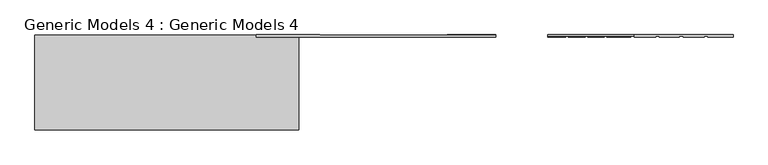
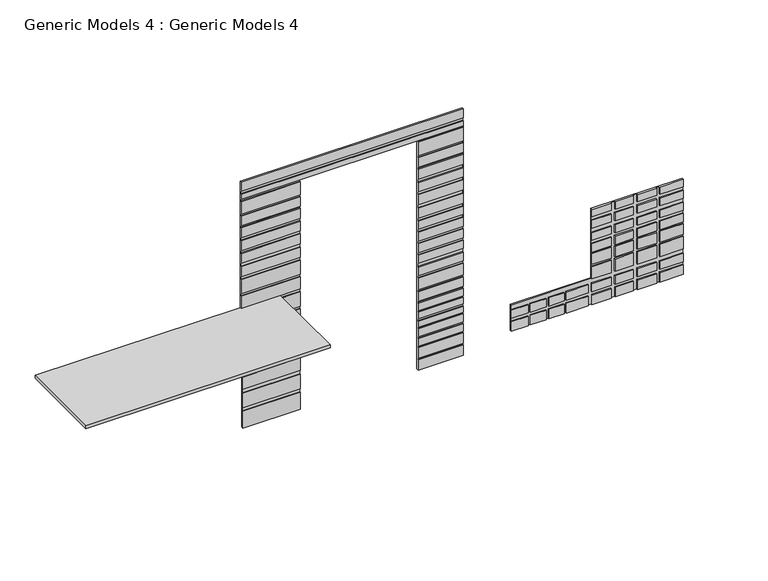
"""IFC4 building model written with IfcOpenShell, lengths in millimetres: proxy geometry, Generic Models 4 : Generic Models 4."""

from ifc_helpers import new_model, si_unit, origin, place, context, project, spatial, faceted_brep, source, transform, mapped, element, save


def generic_models_4_generic_models_4_6a6385c3(model_context):
    return source(origin(), model_context, "Body", "Brep", [
        faceted_brep([(-5873.014323, -13904.9538163, 2677.4848502), (-5873.014323, -13904.9538163, 2489.9387653), (-5393.446906, -13904.9538163, 2489.9387653), (-5393.446906, -13904.9538163, 2677.4848502), (-5873.014323, -13904.9538163, 2393.7857703), (-5873.014323, -13904.9538163, 2187.7436382), (-5393.446906, -13904.9538163, 2187.7436382), (-5393.446906, -13904.9538163, 2393.7857703), (-5873.014323, -13904.9538163, 2077.854501), (-5873.014323, -13904.9538163, 1876.5546729), (-5393.446906, -13904.9538163, 1876.5546729), (-5393.446906, -13904.9538163, 2077.854501), (-5873.014323, -13904.9538163, 1789.395516), (-5873.014323, -13904.9538163, 1569.6172418), (-5393.446906, -13904.9538163, 1569.6172418), (-5393.446906, -13904.9538163, 1789.395516), (-5873.014323, -13904.9538163, 1193.0039496), (-5873.014323, -13904.9538163, 872.4244956), (-5393.446906, -13904.9538163, 872.4244956), (-5393.446906, -13904.9538163, 1193.0039496), (-5873.014323, -13904.9538163, 1524.0), (-5873.014323, -13904.9538163, 1250.1296825), (-5393.446906, -13904.9538163, 1250.1296825), (-5393.446906, -13904.9538163, 1524.0), (-7854.214323, -13904.9538163, 455.5626701), (-7854.214323, -13904.9538163, 207.9039867), (-7441.5943921, -13904.9538163, 207.9039867), (-7441.5943921, -13904.9538163, 455.5626701), (-7854.214323, -13904.9538163, 753.9093053), (-7854.214323, -13904.9538163, 540.1642411), (-7441.5943921, -13904.9538163, 540.1642411), (-7441.5943921, -13904.9538163, 753.9093053), (-3625.114323, -13904.9538163, 2489.9387653), (-3625.114323, -13904.9538163, 2677.4848502), (-4204.9719989, -13904.9538163, 2677.4848502), (-4204.9719989, -13904.9538163, 2489.9387653), (-3625.114323, -13904.9538163, 2187.7436382), (-3625.114323, -13904.9538163, 2393.7857703), (-4204.9719989, -13904.9538163, 2393.7857703), (-4204.9719989, -13904.9538163, 2187.7436382), (-3625.114323, -13904.9538163, 1876.5546729), (-3625.114323, -13904.9538163, 2077.854501), (-4204.9719989, -13904.9538163, 2077.854501), (-4204.9719989, -13904.9538163, 1876.5546729), (-3625.114323, -13904.9538163, 1569.6172418), (-3625.114323, -13904.9538163, 1789.395516), (-4204.9719989, -13904.9538163, 1789.395516), (-4204.9719989, -13904.9538163, 1569.6172418), (-3625.114323, -13904.9538163, 872.4244956), (-3625.114323, -13904.9538163, 1193.0039496), (-4204.9719989, -13904.9538163, 1193.0039496), (-4204.9719989, -13904.9538163, 872.4244956), (-3625.114323, -13904.9538163, 1250.1296825), (-3625.114323, -13904.9538163, 1524.0), (-4204.9719989, -13904.9538163, 1524.0), (-4204.9719989, -13904.9538163, 1250.1296825), (-3625.114323, -13904.9538163, 207.9039867), (-3625.114323, -13904.9538163, 455.5626701), (-4204.9719989, -13904.9538163, 455.5626701), (-4204.9719989, -13904.9538163, 207.9039867), (-3625.114323, -13904.9538163, 540.1642411), (-3625.114323, -13904.9538163, 753.9093053), (-4204.9719989, -13904.9538163, 753.9093053), (-4204.9719989, -13904.9538163, 540.1642411), (-4855.9456918, -13904.9538163, 2677.4848502), (-5303.8633703, -13904.9538163, 2677.4848502), (-5303.8633703, -13904.9538163, 2489.9387653), (-4855.9456918, -13904.9538163, 2489.9387653), (-4282.6110632, -13904.9538163, 2677.4848502), (-4760.3899203, -13904.9538163, 2677.4848502), (-4760.3899203, -13904.9538163, 2489.9387653), (-4282.6110632, -13904.9538163, 2489.9387653), (-5303.8633703, -13904.9538163, 207.9039867), (-4855.9456918, -13904.9538163, 207.9039867), (-4855.9456918, -13904.9538163, 455.5626701), (-5303.8633703, -13904.9538163, 455.5626701), (-4760.3899203, -13904.9538163, 207.9039867), (-4282.6110632, -13904.9538163, 207.9039867), (-4282.6110632, -13904.9538163, 455.5626701), (-4760.3899203, -13904.9538163, 455.5626701), (-5873.014323, -13904.9538163, 207.9039867), (-5393.446906, -13904.9538163, 207.9039867), (-5393.446906, -13904.9538163, 455.5626701), (-5873.014323, -13904.9538163, 455.5626701), (-6501.664323, -13904.9538163, 207.9039867), (-5956.9143625, -13904.9538163, 207.9039867), (-5956.9143625, -13904.9538163, 455.5626701), (-6501.664323, -13904.9538163, 455.5626701), (-6935.8171521, -13904.9538163, 207.9039867), (-6556.6805641, -13904.9538163, 207.9039867), (-6556.6805641, -13904.9538163, 455.5626701), (-6935.8171521, -13904.9538163, 455.5626701), (-7382.8881053, -13904.9538163, 207.9039867), (-6999.0393071, -13904.9538163, 207.9039867), (-6999.0393071, -13904.9538163, 455.5626701), (-7382.8881053, -13904.9538163, 455.5626701), (-5303.8633703, -13904.9538163, 2187.7436382), (-4855.9456918, -13904.9538163, 2187.7436382), (-4855.9456918, -13904.9538163, 2393.7857703), (-5303.8633703, -13904.9538163, 2393.7857703), (-4760.3899203, -13904.9538163, 2187.7436382), (-4282.6110632, -13904.9538163, 2187.7436382), (-4282.6110632, -13904.9538163, 2393.7857703), (-4760.3899203, -13904.9538163, 2393.7857703), (-5303.8633703, -13904.9538163, 1876.5546729), (-4855.9456918, -13904.9538163, 1876.5546729), (-4855.9456918, -13904.9538163, 2077.854501), (-5303.8633703, -13904.9538163, 2077.854501), (-4760.3899203, -13904.9538163, 1876.5546729), (-4282.6110632, -13904.9538163, 1876.5546729), (-4282.6110632, -13904.9538163, 2077.854501), (-4760.3899203, -13904.9538163, 2077.854501), (-5303.8633703, -13904.9538163, 1569.6172418), (-4855.9456918, -13904.9538163, 1569.6172418), (-4855.9456918, -13904.9538163, 1789.395516), (-5303.8633703, -13904.9538163, 1789.395516), (-4760.3899203, -13904.9538163, 1569.6172418), (-4282.6110632, -13904.9538163, 1569.6172418), (-4282.6110632, -13904.9538163, 1789.395516), (-4760.3899203, -13904.9538163, 1789.395516), (-5303.8633703, -13904.9538163, 872.4244956), (-4855.9456918, -13904.9538163, 872.4244956), (-4855.9456918, -13904.9538163, 1193.0039496), (-5303.8633703, -13904.9538163, 1193.0039496), (-4760.3899203, -13904.9538163, 872.4244956), (-4282.6110632, -13904.9538163, 872.4244956), (-4282.6110632, -13904.9538163, 1193.0039496), (-4760.3899203, -13904.9538163, 1193.0039496), (-5303.8633703, -13904.9538163, 1250.1296825), (-4855.9456918, -13904.9538163, 1250.1296825), (-4855.9456918, -13904.9538163, 1524.0), (-5303.8633703, -13904.9538163, 1524.0), (-4760.3899203, -13904.9538163, 1250.1296825), (-4282.6110632, -13904.9538163, 1250.1296825), (-4282.6110632, -13904.9538163, 1524.0), (-4760.3899203, -13904.9538163, 1524.0), (-5303.8633703, -13904.9538163, 540.1642411), (-4855.9456918, -13904.9538163, 540.1642411), (-4855.9456918, -13904.9538163, 753.9093053), (-5303.8633703, -13904.9538163, 753.9093053), (-4760.3899203, -13904.9538163, 540.1642411), (-4282.6110632, -13904.9538163, 540.1642411), (-4282.6110632, -13904.9538163, 753.9093053), (-4760.3899203, -13904.9538163, 753.9093053), (-5873.014323, -13904.9538163, 540.1642411), (-5393.446906, -13904.9538163, 540.1642411), (-5393.446906, -13904.9538163, 753.9093053), (-5873.014323, -13904.9538163, 753.9093053), (-6501.664323, -13904.9538163, 540.1642411), (-5956.9143625, -13904.9538163, 540.1642411), (-5956.9143625, -13904.9538163, 753.9093053), (-6501.664323, -13904.9538163, 753.9093053), (-6935.8171521, -13904.9538163, 540.1642411), (-6556.6805641, -13904.9538163, 540.1642411), (-6556.6805641, -13904.9538163, 753.9093053), (-6935.8171521, -13904.9538163, 753.9093053), (-7382.8881053, -13904.9538163, 540.1642411), (-6999.0393071, -13904.9538163, 540.1642411), (-6999.0393071, -13904.9538163, 753.9093053), (-7382.8881053, -13904.9538163, 753.9093053), (-3625.114323, -13854.1538163, 2677.4848502), (-3625.114323, -13854.1538163, 207.9039867), (-7854.214323, -13854.1538163, 207.9039867), (-7854.214323, -13854.1538163, 872.4244956), (-5873.014323, -13854.1538163, 872.4244956), (-5873.014323, -13854.1538163, 2677.4848502), (-5393.446906, -13879.5538163, 2677.4848502), (-5303.8633703, -13879.5538163, 2677.4848502), (-4855.9456918, -13879.5538163, 2677.4848502), (-4760.3899203, -13879.5538163, 2677.4848502), (-4282.6110632, -13879.5538163, 2677.4848502), (-4204.9719989, -13879.5538163, 2677.4848502), (-5873.014323, -13879.5538163, 872.4244956), (-5873.014323, -13879.5538163, 1193.0039496), (-5873.014323, -13879.5538163, 1250.1296825), (-5873.014323, -13879.5538163, 1524.0), (-5873.014323, -13879.5538163, 1569.6172418), (-5873.014323, -13879.5538163, 1789.395516), (-5873.014323, -13879.5538163, 1876.5546729), (-5873.014323, -13879.5538163, 2077.854501), (-5873.014323, -13879.5538163, 2187.7436382), (-5873.014323, -13879.5538163, 2393.7857703), (-5873.014323, -13879.5538163, 2489.9387653), (-4204.9719989, -13879.5538163, 207.9039867), (-4282.6110632, -13879.5538163, 207.9039867), (-4760.3899203, -13879.5538163, 207.9039867), (-4855.9456918, -13879.5538163, 207.9039867), (-5303.8633703, -13879.5538163, 207.9039867), (-5393.446906, -13879.5538163, 207.9039867), (-5873.014323, -13879.5538163, 207.9039867), (-5956.9143625, -13879.5538163, 207.9039867), (-6501.664323, -13879.5538163, 207.9039867), (-6556.6805641, -13879.5538163, 207.9039867), (-6935.8171521, -13879.5538163, 207.9039867), (-6999.0393071, -13879.5538163, 207.9039867), (-7382.8881053, -13879.5538163, 207.9039867), (-7441.5943921, -13879.5538163, 207.9039867), (-3625.114323, -13879.5538163, 2489.9387653), (-3625.114323, -13879.5538163, 2393.7857703), (-3625.114323, -13879.5538163, 2187.7436382), (-3625.114323, -13879.5538163, 2077.854501), (-3625.114323, -13879.5538163, 1876.5546729), (-3625.114323, -13879.5538163, 1789.395516), (-3625.114323, -13879.5538163, 1569.6172418), (-3625.114323, -13879.5538163, 1524.0), (-3625.114323, -13879.5538163, 1250.1296825), (-3625.114323, -13879.5538163, 1193.0039496), (-3625.114323, -13879.5538163, 872.4244956), (-3625.114323, -13879.5538163, 753.9093053), (-3625.114323, -13879.5538163, 540.1642411), (-3625.114323, -13879.5538163, 455.5626701), (-7854.214323, -13879.5538163, 455.5626701), (-7854.214323, -13879.5538163, 540.1642411), (-7854.214323, -13879.5538163, 753.9093053), (-7854.214323, -13879.5538163, 872.4244956), (-5393.446906, -13879.5538163, 2393.7857703), (-5393.446906, -13879.5538163, 2187.7436382), (-5393.446906, -13879.5538163, 2077.854501), (-5393.446906, -13879.5538163, 1876.5546729), (-5393.446906, -13879.5538163, 1789.395516), (-5393.446906, -13879.5538163, 1569.6172418), (-5393.446906, -13879.5538163, 1524.0), (-5393.446906, -13879.5538163, 1250.1296825), (-5393.446906, -13879.5538163, 1193.0039496), (-5393.446906, -13879.5538163, 872.4244956), (-7441.5943921, -13879.5538163, 753.9093053), (-7441.5943921, -13879.5538163, 540.1642411), (-7441.5943921, -13879.5538163, 455.5626701), (-7382.8881053, -13879.5538163, 455.5626701), (-6999.0393071, -13879.5538163, 455.5626701), (-6935.8171521, -13879.5538163, 455.5626701), (-6556.6805641, -13879.5538163, 455.5626701), (-6501.664323, -13879.5538163, 455.5626701), (-5956.9143625, -13879.5538163, 455.5626701), (-5873.014323, -13879.5538163, 455.5626701), (-5393.446906, -13879.5538163, 455.5626701), (-5303.8633703, -13879.5538163, 455.5626701), (-4855.9456918, -13879.5538163, 455.5626701), (-4760.3899203, -13879.5538163, 455.5626701), (-4282.6110632, -13879.5538163, 455.5626701), (-4204.9719989, -13879.5538163, 455.5626701), (-4204.9719989, -13879.5538163, 540.1642411), (-4204.9719989, -13879.5538163, 753.9093053), (-4204.9719989, -13879.5538163, 872.4244956), (-4204.9719989, -13879.5538163, 1193.0039496), (-4204.9719989, -13879.5538163, 1250.1296825), (-4204.9719989, -13879.5538163, 1524.0), (-4204.9719989, -13879.5538163, 1569.6172418), (-4204.9719989, -13879.5538163, 1789.395516), (-4204.9719989, -13879.5538163, 1876.5546729), (-4204.9719989, -13879.5538163, 2077.854501), (-4204.9719989, -13879.5538163, 2187.7436382), (-4204.9719989, -13879.5538163, 2393.7857703), (-4204.9719989, -13879.5538163, 2489.9387653), (-4282.6110632, -13879.5538163, 2489.9387653), (-4760.3899203, -13879.5538163, 2489.9387653), (-4855.9456918, -13879.5538163, 2489.9387653), (-5303.8633703, -13879.5538163, 2489.9387653), (-5393.446906, -13879.5538163, 2489.9387653), (-5303.8633703, -13879.5538163, 2393.7857703), (-4855.9456918, -13879.5538163, 2393.7857703), (-4855.9456918, -13879.5538163, 2187.7436382), (-5303.8633703, -13879.5538163, 2187.7436382), (-4760.3899203, -13879.5538163, 2393.7857703), (-4282.6110632, -13879.5538163, 2393.7857703), (-4282.6110632, -13879.5538163, 2187.7436382), (-4760.3899203, -13879.5538163, 2187.7436382), (-5303.8633703, -13879.5538163, 2077.854501), (-4855.9456918, -13879.5538163, 2077.854501), (-4855.9456918, -13879.5538163, 1876.5546729), (-5303.8633703, -13879.5538163, 1876.5546729), (-4760.3899203, -13879.5538163, 2077.854501), (-4282.6110632, -13879.5538163, 2077.854501), (-4282.6110632, -13879.5538163, 1876.5546729), (-4760.3899203, -13879.5538163, 1876.5546729), (-5303.8633703, -13879.5538163, 1789.395516), (-4855.9456918, -13879.5538163, 1789.395516), (-4855.9456918, -13879.5538163, 1569.6172418), (-5303.8633703, -13879.5538163, 1569.6172418), (-4760.3899203, -13879.5538163, 1789.395516), (-4282.6110632, -13879.5538163, 1789.395516), (-4282.6110632, -13879.5538163, 1569.6172418), (-4760.3899203, -13879.5538163, 1569.6172418), (-5303.8633703, -13879.5538163, 1524.0), (-4855.9456918, -13879.5538163, 1524.0), (-4855.9456918, -13879.5538163, 1250.1296825), (-5303.8633703, -13879.5538163, 1250.1296825), (-4760.3899203, -13879.5538163, 1524.0), (-4282.6110632, -13879.5538163, 1524.0), (-4282.6110632, -13879.5538163, 1250.1296825), (-4760.3899203, -13879.5538163, 1250.1296825), (-5303.8633703, -13879.5538163, 753.9093053), (-4855.9456918, -13879.5538163, 753.9093053), (-4855.9456918, -13879.5538163, 540.1642411), (-5303.8633703, -13879.5538163, 540.1642411), (-4760.3899203, -13879.5538163, 753.9093053), (-4282.6110632, -13879.5538163, 753.9093053), (-4282.6110632, -13879.5538163, 540.1642411), (-4760.3899203, -13879.5538163, 540.1642411), (-5873.014323, -13879.5538163, 753.9093053), (-5393.446906, -13879.5538163, 753.9093053), (-5393.446906, -13879.5538163, 540.1642411), (-5873.014323, -13879.5538163, 540.1642411), (-6501.664323, -13879.5538163, 753.9093053), (-5956.9143625, -13879.5538163, 753.9093053), (-5956.9143625, -13879.5538163, 540.1642411), (-6501.664323, -13879.5538163, 540.1642411), (-6935.8171521, -13879.5538163, 753.9093053), (-6556.6805641, -13879.5538163, 753.9093053), (-6556.6805641, -13879.5538163, 540.1642411), (-6935.8171521, -13879.5538163, 540.1642411), (-7382.8881053, -13879.5538163, 753.9093053), (-6999.0393071, -13879.5538163, 753.9093053), (-6999.0393071, -13879.5538163, 540.1642411), (-7382.8881053, -13879.5538163, 540.1642411), (-5303.8633703, -13879.5538163, 1193.0039496), (-4855.9456918, -13879.5538163, 1193.0039496), (-4855.9456918, -13879.5538163, 872.4244956), (-5303.8633703, -13879.5538163, 872.4244956), (-4760.3899203, -13879.5538163, 1193.0039496), (-4282.6110632, -13879.5538163, 1193.0039496), (-4282.6110632, -13879.5538163, 872.4244956), (-4760.3899203, -13879.5538163, 872.4244956)], [[[0, 1, 2, 3]], [[4, 5, 6, 7]], [[8, 9, 10, 11]], [[12, 13, 14, 15]], [[16, 17, 18, 19]], [[20, 21, 22, 23]], [[24, 25, 26, 27]], [[28, 29, 30, 31]], [[32, 33, 34, 35]], [[36, 37, 38, 39]], [[40, 41, 42, 43]], [[44, 45, 46, 47]], [[48, 49, 50, 51]], [[52, 53, 54, 55]], [[56, 57, 58, 59]], [[60, 61, 62, 63]], [[64, 65, 66, 67]], [[68, 69, 70, 71]], [[72, 73, 74, 75]], [[76, 77, 78, 79]], [[80, 81, 82, 83]], [[84, 85, 86, 87]], [[88, 89, 90, 91]], [[92, 93, 94, 95]], [[96, 97, 98, 99]], [[100, 101, 102, 103]], [[104, 105, 106, 107]], [[108, 109, 110, 111]], [[112, 113, 114, 115]], [[116, 117, 118, 119]], [[120, 121, 122, 123]], [[124, 125, 126, 127]], [[128, 129, 130, 131]], [[132, 133, 134, 135]], [[136, 137, 138, 139]], [[140, 141, 142, 143]], [[144, 145, 146, 147]], [[148, 149, 150, 151]], [[152, 153, 154, 155]], [[156, 157, 158, 159]], [[160, 161, 162, 163, 164, 165]], [[160, 165, 0, 3, 166, 167, 65, 64, 168, 169, 69, 68, 170, 171, 34, 33]], [[0, 165, 164, 172, 17, 16, 173, 174, 21, 20, 175, 176, 13, 12, 177, 178, 9, 8, 179, 180, 5, 4, 181, 182, 1]], [[161, 56, 59, 183, 184, 77, 76, 185, 186, 73, 72, 187, 188, 81, 80, 189, 190, 85, 84, 191, 192, 89, 88, 193, 194, 93, 92, 195, 196, 26, 25, 162]], [[161, 160, 33, 32, 197, 198, 37, 36, 199, 200, 41, 40, 201, 202, 45, 44, 203, 204, 53, 52, 205, 206, 49, 48, 207, 208, 61, 60, 209, 210, 57, 56]], [[163, 162, 25, 24, 211, 212, 29, 28, 213, 214]], [[164, 163, 214, 172]], [[182, 181, 215, 216, 180, 179, 217, 218, 178, 177, 219, 220, 176, 175, 221, 222, 174, 173, 223, 224, 172, 214, 213, 225, 226, 212, 211, 227, 196, 195, 228, 229, 194, 193, 230, 231, 192, 191, 232, 233, 190, 189, 234, 235, 188, 187, 236, 237, 186, 185, 238, 239, 184, 183, 240, 210, 209, 241, 242, 208, 207, 243, 244, 206, 205, 245, 246, 204, 203, 247, 248, 202, 201, 249, 250, 200, 199, 251, 252, 198, 197, 253, 171, 170, 254, 255, 169, 168, 256, 257, 167, 166, 258], [259, 260, 261, 262], [263, 264, 265, 266], [267, 268, 269, 270], [271, 272, 273, 274], [275, 276, 277, 278], [279, 280, 281, 282], [283, 284, 285, 286], [287, 288, 289, 290], [291, 292, 293, 294], [295, 296, 297, 298], [299, 300, 301, 302], [303, 304, 305, 306], [307, 308, 309, 310], [311, 312, 313, 314], [315, 316, 317, 318], [319, 320, 321, 322]], [[99, 98, 260, 259]], [[103, 102, 264, 263]], [[181, 4, 7, 215]], [[37, 198, 252, 38]], [[67, 66, 257, 256]], [[71, 70, 255, 254]], [[1, 182, 258, 2]], [[197, 32, 35, 253]], [[107, 106, 268, 267]], [[111, 110, 272, 271]], [[179, 8, 11, 217]], [[41, 200, 250, 42]], [[97, 96, 262, 261]], [[101, 100, 266, 265]], [[5, 180, 216, 6]], [[199, 36, 39, 251]], [[115, 114, 276, 275]], [[119, 118, 280, 279]], [[177, 12, 15, 219]], [[45, 202, 248, 46]], [[105, 104, 270, 269]], [[109, 108, 274, 273]], [[9, 178, 218, 10]], [[201, 40, 43, 249]], [[131, 130, 284, 283]], [[135, 134, 288, 287]], [[175, 20, 23, 221]], [[53, 204, 246, 54]], [[113, 112, 278, 277]], [[117, 116, 282, 281]], [[13, 176, 220, 14]], [[203, 44, 47, 247]], [[139, 138, 292, 291]], [[143, 142, 296, 295]], [[147, 146, 300, 299]], [[151, 150, 304, 303]], [[155, 154, 308, 307]], [[159, 158, 312, 311]], [[61, 208, 242, 62]], [[213, 28, 31, 225]], [[121, 120, 318, 317]], [[125, 124, 322, 321]], [[17, 172, 224, 18]], [[207, 48, 51, 243]], [[123, 122, 316, 315]], [[127, 126, 320, 319]], [[173, 16, 19, 223]], [[49, 206, 244, 50]], [[129, 128, 286, 285]], [[133, 132, 290, 289]], [[21, 174, 222, 22]], [[205, 52, 55, 245]], [[75, 74, 237, 236]], [[79, 78, 239, 238]], [[83, 82, 235, 234]], [[87, 86, 233, 232]], [[91, 90, 231, 230]], [[95, 94, 229, 228]], [[57, 210, 240, 58]], [[211, 24, 27, 227]], [[137, 136, 294, 293]], [[141, 140, 298, 297]], [[145, 144, 302, 301]], [[149, 148, 306, 305]], [[153, 152, 310, 309]], [[157, 156, 314, 313]], [[209, 60, 63, 241]], [[29, 212, 226, 30]], [[236, 187, 72, 75]], [[167, 257, 66, 65]], [[259, 262, 96, 99]], [[267, 270, 104, 107]], [[275, 278, 112, 115]], [[283, 286, 128, 131]], [[291, 294, 136, 139]], [[315, 318, 120, 123]], [[216, 215, 7, 6]], [[218, 217, 11, 10]], [[220, 219, 15, 14]], [[222, 221, 23, 22]], [[224, 223, 19, 18]], [[188, 235, 82, 81]], [[258, 166, 3, 2]], [[301, 300, 146, 145]], [[238, 185, 76, 79]], [[169, 255, 70, 69]], [[263, 266, 100, 103]], [[271, 274, 108, 111]], [[279, 282, 116, 119]], [[287, 290, 132, 135]], [[295, 298, 140, 143]], [[319, 322, 124, 127]], [[186, 237, 74, 73]], [[256, 168, 64, 67]], [[261, 260, 98, 97]], [[269, 268, 106, 105]], [[277, 276, 114, 113]], [[285, 284, 130, 129]], [[293, 292, 138, 137]], [[317, 316, 122, 121]], [[240, 183, 59, 58]], [[242, 241, 63, 62]], [[244, 243, 51, 50]], [[246, 245, 55, 54]], [[248, 247, 47, 46]], [[250, 249, 43, 42]], [[252, 251, 39, 38]], [[171, 253, 35, 34]], [[184, 239, 78, 77]], [[254, 170, 68, 71]], [[265, 264, 102, 101]], [[273, 272, 110, 109]], [[281, 280, 118, 117]], [[289, 288, 134, 133]], [[297, 296, 142, 141]], [[321, 320, 126, 125]], [[234, 189, 80, 83]], [[299, 302, 144, 147]], [[190, 233, 86, 85]], [[305, 304, 150, 149]], [[232, 191, 84, 87]], [[303, 306, 148, 151]], [[192, 231, 90, 89]], [[309, 308, 154, 153]], [[230, 193, 88, 91]], [[307, 310, 152, 155]], [[194, 229, 94, 93]], [[313, 312, 158, 157]], [[228, 195, 92, 95]], [[311, 314, 156, 159]], [[226, 225, 31, 30]], [[196, 227, 27, 26]]]),
        faceted_brep([(-19541.0149344, -16025.8538163, 3124.2), (-13531.114323, -16025.8538163, 3124.2), (-13531.114323, -13904.9538163, 3124.2), (-13531.114323, -13879.5538163, 3124.2), (-13531.114323, -13864.3466243, 3124.2), (-19541.0149344, -13864.3466243, 3124.2), (-19541.0149344, -16025.8538163, 3048.0), (-19541.0149344, -13864.3466243, 3048.0), (-13531.114323, -13864.3466243, 3048.0), (-13531.114323, -13879.5538163, 3048.0), (-13531.114323, -13904.9538163, 3048.0), (-13531.114323, -16025.8538163, 3048.0)], [[[0, 1, 2, 3, 4, 5]], [[6, 7, 8, 9, 10, 11]], [[1, 0, 6, 11]], [[1, 11, 10, 9, 8, 4, 3, 2]], [[5, 4, 8, 7]], [[0, 5, 7, 6]]]),
        faceted_brep([(-10145.5548754, -13904.9538163, 0.0), (-9031.8508279, -13904.9538163, 0.0), (-9031.8508279, -13904.9538163, 271.2389196), (-10145.5548754, -13904.9538163, 271.2389196), (-14456.9434854, -13904.9538163, 0.0), (-13042.1380521, -13904.9538163, 0.0), (-13042.1380521, -13904.9538163, 435.4628413), (-14456.9434854, -13904.9538163, 435.4628413), (-9034.7947562, -13904.9538163, 6400.8), (-14496.314323, -13904.9538163, 6400.8), (-14496.314323, -13904.9538163, 6174.9916024), (-9034.7947562, -13904.9538163, 6174.9916024), (-14456.9434854, -13904.9538163, 2603.4282114), (-14456.9434854, -13904.9538163, 2323.2410122), (-13042.1380521, -13904.9538163, 2323.2410122), (-13042.1380521, -13904.9538163, 2603.4282114), (-14456.9434854, -13904.9538163, 2214.2447243), (-14456.9434854, -13904.9538163, 1896.3388846), (-13042.1380521, -13904.9538163, 1896.3388846), (-13042.1380521, -13904.9538163, 2214.2447243), (-14456.9434854, -13904.9538163, 1796.2367487), (-14456.9434854, -13904.9538163, 1439.097053), (-13042.1380521, -13904.9538163, 1439.097053), (-13042.1380521, -13904.9538163, 1796.2367487), (-14456.9434854, -13904.9538163, 1329.2079159), (-14456.9434854, -13904.9538163, 1006.4085756), (-13042.1380521, -13904.9538163, 1006.4085756), (-13042.1380521, -13904.9538163, 1329.2079159), (-14456.9434854, -13904.9538163, 901.297227), (-14456.9434854, -13904.9538163, 525.046377), (-13042.1380521, -13904.9538163, 525.046377), (-13042.1380521, -13904.9538163, 901.297227), (-13042.1380521, -13904.9538163, 5572.0332004), (-13042.1380521, -13904.9538163, 5906.3837859), (-14496.314323, -13904.9538163, 5906.3837859), (-14496.314323, -13904.9538163, 5572.0332004), (-13042.1380521, -13904.9538163, 5272.8451776), (-13042.1380521, -13904.9538163, 5516.7491981), (-14496.314323, -13904.9538163, 5516.7491981), (-14496.314323, -13904.9538163, 5272.8451776), (-13042.1380521, -13904.9538163, 4959.8164826), (-13042.1380521, -13904.9538163, 5227.6864954), (-14496.314323, -13904.9538163, 5227.6864954), (-14496.314323, -13904.9538163, 4959.8164826), (-13042.1380521, -13904.9538163, 4631.3435183), (-13042.1380521, -13904.9538163, 4888.149654), (-14496.314323, -13904.9538163, 4888.149654), (-14496.314323, -13904.9538163, 4631.3435183), (-13042.1380521, -13904.9538163, 4302.8705541), (-13042.1380521, -13904.9538163, 4553.704454), (-14496.314323, -13904.9538163, 4553.704454), (-14496.314323, -13904.9538163, 4302.8705541), (-13042.1380521, -13904.9538163, 3944.5364112), (-13042.1380521, -13904.9538163, 4204.113055), (-14496.314323, -13904.9538163, 4204.113055), (-14496.314323, -13904.9538163, 3944.5364112), (-13042.1380521, -13904.9538163, 3506.7585502), (-13042.1380521, -13904.9538163, 3868.9746463), (-14496.314323, -13904.9538163, 3868.9746463), (-14496.314323, -13904.9538163, 3506.7585502), (-10145.5548754, -13904.9538163, 3279.1839932), (-10145.5548754, -13904.9538163, 3048.0), (-9031.8508279, -13904.9538163, 3048.0), (-9031.8508279, -13904.9538163, 3279.1839932), (-10145.5548754, -13904.9538163, 2980.5722075), (-10145.5548754, -13904.9538163, 2777.5161932), (-9031.8508279, -13904.9538163, 2777.5161932), (-9031.8508279, -13904.9538163, 2980.5722075), (-10145.5548754, -13904.9538163, 2678.7342332), (-10145.5548754, -13904.9538163, 2450.5872675), (-9031.8508279, -13904.9538163, 2450.5872675), (-9031.8508279, -13904.9538163, 2678.7342332), (-10145.5548754, -13904.9538163, 2385.7845586), (-10145.5548754, -13904.9538163, 2086.8248817), (-9031.8508279, -13904.9538163, 2086.8248817), (-9031.8508279, -13904.9538163, 2385.7845586), (-10145.5548754, -13904.9538163, 2040.4206102), (-10145.5548754, -13904.9538163, 1796.2367487), (-9031.8508279, -13904.9538163, 1796.2367487), (-9031.8508279, -13904.9538163, 2040.4206102), (-10145.5548754, -13904.9538163, 1743.4119577), (-10145.5548754, -13904.9538163, 1544.7137562), (-9031.8508279, -13904.9538163, 1544.7137562), (-9031.8508279, -13904.9538163, 1743.4119577), (-10145.5548754, -13904.9538163, 1499.5550741), (-10145.5548754, -13904.9538163, 1329.2079159), (-9031.8508279, -13904.9538163, 1329.2079159), (-9031.8508279, -13904.9538163, 1499.5550741), (-10145.5548754, -13904.9538163, 1273.7616633), (-10145.5548754, -13904.9538163, 1120.222144), (-9031.8508279, -13904.9538163, 1120.222144), (-9031.8508279, -13904.9538163, 1273.7616633), (-10145.5548754, -13904.9538163, 1075.0634619), (-10145.5548754, -13904.9538163, 872.4244956), (-9031.8508279, -13904.9538163, 872.4244956), (-9031.8508279, -13904.9538163, 1075.0634619), (-10145.5548754, -13904.9538163, 813.1431054), (-10145.5548754, -13904.9538163, 618.9607722), (-9031.8508279, -13904.9538163, 618.9607722), (-9031.8508279, -13904.9538163, 813.1431054), (-10145.5548754, -13904.9538163, 578.3179583), (-10145.5548754, -13904.9538163, 311.8817336), (-9031.8508279, -13904.9538163, 311.8817336), (-9031.8508279, -13904.9538163, 578.3179583), (-13042.1380521, -13904.9538163, 3048.0), (-13736.7607506, -13904.9538163, 3048.0), (-13736.7607506, -13904.9538163, 2678.7342332), (-13042.1380521, -13904.9538163, 2678.7342332), (-14496.314323, -13904.9538163, 3124.2), (-13042.1380521, -13904.9538163, 3124.2), (-13042.1380521, -13904.9538163, 3438.0778395), (-14496.314323, -13904.9538163, 3438.0778395), (-14496.314323, -13904.9538163, 5963.9849303), (-9034.7947562, -13904.9538163, 5963.9849303), (-9034.7947562, -13904.9538163, 5920.582434), (-10145.5548754, -13904.9538163, 5920.582434), (-10145.5548754, -13904.9538163, 5572.0332004), (-9034.7947562, -13904.9538163, 5572.0332004), (-9034.7947562, -13904.9538163, 5516.7491981), (-10145.5548754, -13904.9538163, 5516.7491981), (-10145.5548754, -13904.9538163, 5272.8451776), (-9034.7947562, -13904.9538163, 5272.8451776), (-9034.7947562, -13904.9538163, 5227.6864954), (-10145.5548754, -13904.9538163, 5227.6864954), (-10145.5548754, -13904.9538163, 4959.8164826), (-9034.7947562, -13904.9538163, 4959.8164826), (-9034.7947562, -13904.9538163, 4876.8), (-10145.5548754, -13904.9538163, 4876.8), (-10145.5548754, -13904.9538163, 4631.3435183), (-9034.7947562, -13904.9538163, 4631.3435183), (-9034.7947562, -13904.9538163, 4553.704454), (-10145.5548754, -13904.9538163, 4553.704454), (-10145.5548754, -13904.9538163, 4302.8705541), (-9034.7947562, -13904.9538163, 4302.8705541), (-9034.7947562, -13904.9538163, 4204.113055), (-10145.5548754, -13904.9538163, 4204.113055), (-10145.5548754, -13904.9538163, 3944.5364112), (-9034.7947562, -13904.9538163, 3944.5364112), (-9034.7947562, -13904.9538163, 3868.9746463), (-10145.5548754, -13904.9538163, 3868.9746463), (-10145.5548754, -13904.9538163, 3667.3793146), (-9034.7947562, -13904.9538163, 3667.3793146), (-9034.7947562, -13904.9538163, 3583.7680146), (-10145.5548754, -13904.9538163, 3583.7680146), (-10145.5548754, -13904.9538163, 3352.8), (-9031.8508279, -13904.9538163, 3352.8), (-9031.8508279, -13904.9538163, 6096.0), (-14496.314323, -13904.9538163, 6096.0), (-13736.7607506, -13854.1538163, 3048.0), (-13531.114323, -13854.1538163, 3048.0), (-13531.114323, -13854.1538163, 3124.2), (-14496.314323, -13854.1538163, 3124.2), (-14496.314323, -13854.1538163, 6400.8), (-13042.1380521, -13854.1538163, 6400.8), (-13042.1380521, -13854.1538163, 0.0), (-14456.9434854, -13854.1538163, 0.0), (-14456.9434854, -13854.1538163, 2678.7342332), (-13736.7607506, -13854.1538163, 2678.7342332), (-9031.8508279, -13854.1538163, 5963.9849303), (-9031.8508279, -13854.1538163, 0.0), (-10145.5548754, -13854.1538163, 0.0), (-10145.5548754, -13854.1538163, 5963.9849303), (-13042.1380521, -13879.5538163, 3048.0), (-13531.114323, -13879.5538163, 3048.0), (-13736.7607506, -13879.5538163, 2678.7342332), (-13531.114323, -13879.5538163, 3124.2), (-13042.1380521, -13864.3466243, 6400.8), (-13042.1380521, -13864.3466243, 5963.9849303), (-13042.1380521, -13879.5538163, 5963.9849303), (-13042.1380521, -13879.5538163, 5906.3837859), (-13042.1380521, -13879.5538163, 5572.0332004), (-13042.1380521, -13879.5538163, 5516.7491981), (-13042.1380521, -13879.5538163, 5272.8451776), (-13042.1380521, -13879.5538163, 5227.6864954), (-13042.1380521, -13879.5538163, 4959.8164826), (-13042.1380521, -13879.5538163, 4888.149654), (-13042.1380521, -13879.5538163, 4631.3435183), (-13042.1380521, -13879.5538163, 4553.704454), (-13042.1380521, -13879.5538163, 4302.8705541), (-13042.1380521, -13879.5538163, 4204.113055), (-13042.1380521, -13879.5538163, 3944.5364112), (-13042.1380521, -13879.5538163, 3868.9746463), (-13042.1380521, -13879.5538163, 3506.7585502), (-13042.1380521, -13879.5538163, 3438.0778395), (-13042.1380521, -13879.5538163, 3124.2), (-13042.1380521, -13879.5538163, 2678.7342332), (-13042.1380521, -13879.5538163, 2603.4282114), (-13042.1380521, -13879.5538163, 2323.2410122), (-13042.1380521, -13879.5538163, 2214.2447243), (-13042.1380521, -13879.5538163, 1896.3388846), (-13042.1380521, -13879.5538163, 1796.2367487), (-13042.1380521, -13879.5538163, 1439.097053), (-13042.1380521, -13879.5538163, 1329.2079159), (-13042.1380521, -13879.5538163, 1006.4085756), (-13042.1380521, -13879.5538163, 901.297227), (-13042.1380521, -13879.5538163, 525.046377), (-13042.1380521, -13879.5538163, 435.4628413), (-9034.7947562, -13864.3466243, 6400.8), (-14496.314323, -13879.5538163, 3438.0778395), (-14496.314323, -13879.5538163, 3506.7585502), (-14496.314323, -13879.5538163, 3868.9746463), (-14496.314323, -13879.5538163, 3944.5364112), (-14496.314323, -13879.5538163, 4204.113055), (-14496.314323, -13879.5538163, 4302.8705541), (-14496.314323, -13879.5538163, 4553.704454), (-14496.314323, -13879.5538163, 4631.3435183), (-14496.314323, -13879.5538163, 4888.149654), (-14496.314323, -13879.5538163, 4959.8164826), (-14496.314323, -13879.5538163, 5227.6864954), (-14496.314323, -13879.5538163, 5272.8451776), (-14496.314323, -13879.5538163, 5516.7491981), (-14496.314323, -13879.5538163, 5572.0332004), (-14496.314323, -13879.5538163, 5906.3837859), (-14496.314323, -13879.5538163, 5963.9849303), (-14496.314323, -13879.5538163, 6096.0), (-14496.314323, -13879.5538163, 6174.9916024), (-10145.5548754, -13864.3466243, 5963.9849303), (-9031.8508279, -13864.3466243, 5963.9849303), (-10145.5548754, -13879.5538163, 271.2389196), (-10145.5548754, -13879.5538163, 311.8817336), (-10145.5548754, -13879.5538163, 578.3179583), (-10145.5548754, -13879.5538163, 618.9607722), (-10145.5548754, -13879.5538163, 813.1431054), (-10145.5548754, -13879.5538163, 872.4244956), (-10145.5548754, -13879.5538163, 1075.0634619), (-10145.5548754, -13879.5538163, 1120.222144), (-10145.5548754, -13879.5538163, 1273.7616633), (-10145.5548754, -13879.5538163, 1329.2079159), (-10145.5548754, -13879.5538163, 1499.5550741), (-10145.5548754, -13879.5538163, 1544.7137562), (-10145.5548754, -13879.5538163, 1743.4119577), (-10145.5548754, -13879.5538163, 1796.2367487), (-10145.5548754, -13879.5538163, 2040.4206102), (-10145.5548754, -13879.5538163, 2086.8248817), (-10145.5548754, -13879.5538163, 2385.7845586), (-10145.5548754, -13879.5538163, 2450.5872675), (-10145.5548754, -13879.5538163, 2678.7342332), (-10145.5548754, -13879.5538163, 2777.5161932), (-10145.5548754, -13879.5538163, 2980.5722075), (-10145.5548754, -13879.5538163, 3048.0), (-10145.5548754, -13879.5538163, 3279.1839932), (-10145.5548754, -13879.5538163, 3352.8), (-10145.5548754, -13879.5538163, 3583.7680146), (-10145.5548754, -13879.5538163, 3667.3793146), (-10145.5548754, -13879.5538163, 3868.9746463), (-10145.5548754, -13879.5538163, 3944.5364112), (-10145.5548754, -13879.5538163, 4204.113055), (-10145.5548754, -13879.5538163, 4302.8705541), (-10145.5548754, -13879.5538163, 4553.704454), (-10145.5548754, -13879.5538163, 4631.3435183), (-10145.5548754, -13879.5538163, 4876.8), (-10145.5548754, -13879.5538163, 4959.8164826), (-10145.5548754, -13879.5538163, 5227.6864954), (-10145.5548754, -13879.5538163, 5272.8451776), (-10145.5548754, -13879.5538163, 5516.7491981), (-10145.5548754, -13879.5538163, 5572.0332004), (-10145.5548754, -13879.5538163, 5920.582434), (-10145.5548754, -13879.5538163, 5963.9849303), (-9031.8508279, -13864.3466243, 6096.0), (-9031.8508279, -13879.5538163, 3352.8), (-9031.8508279, -13879.5538163, 3279.1839932), (-9031.8508279, -13879.5538163, 3048.0), (-9031.8508279, -13879.5538163, 2980.5722075), (-9031.8508279, -13879.5538163, 2777.5161932), (-9031.8508279, -13879.5538163, 2678.7342332), (-9031.8508279, -13879.5538163, 2450.5872675), (-9031.8508279, -13879.5538163, 2385.7845586), (-9031.8508279, -13879.5538163, 2086.8248817), (-9031.8508279, -13879.5538163, 2040.4206102), (-9031.8508279, -13879.5538163, 1796.2367487), (-9031.8508279, -13879.5538163, 1743.4119577), (-9031.8508279, -13879.5538163, 1544.7137562), (-9031.8508279, -13879.5538163, 1499.5550741), (-9031.8508279, -13879.5538163, 1329.2079159), (-9031.8508279, -13879.5538163, 1273.7616633), (-9031.8508279, -13879.5538163, 1120.222144), (-9031.8508279, -13879.5538163, 1075.0634619), (-9031.8508279, -13879.5538163, 872.4244956), (-9031.8508279, -13879.5538163, 813.1431054), (-9031.8508279, -13879.5538163, 618.9607722), (-9031.8508279, -13879.5538163, 578.3179583), (-9031.8508279, -13879.5538163, 311.8817336), (-9031.8508279, -13879.5538163, 271.2389196), (-14456.9434854, -13879.5538163, 435.4628413), (-14456.9434854, -13879.5538163, 525.046377), (-14456.9434854, -13879.5538163, 901.297227), (-14456.9434854, -13879.5538163, 1006.4085756), (-14456.9434854, -13879.5538163, 1329.2079159), (-14456.9434854, -13879.5538163, 1439.097053), (-14456.9434854, -13879.5538163, 1796.2367487), (-14456.9434854, -13879.5538163, 1896.3388846), (-14456.9434854, -13879.5538163, 2214.2447243), (-14456.9434854, -13879.5538163, 2323.2410122), (-14456.9434854, -13879.5538163, 2603.4282114), (-14456.9434854, -13879.5538163, 2678.7342332), (-9034.7947562, -13864.3466243, 6096.0), (-9034.7947562, -13879.5538163, 6174.9916024), (-9034.7947562, -13879.5538163, 6096.0), (-9034.7947562, -13879.5538163, 5963.9849303), (-9034.7947562, -13879.5538163, 5920.582434), (-9034.7947562, -13879.5538163, 5572.0332004), (-9034.7947562, -13879.5538163, 5516.7491981), (-9034.7947562, -13879.5538163, 4959.8164826), (-9034.7947562, -13879.5538163, 4876.8), (-9034.7947562, -13879.5538163, 5272.8451776), (-9034.7947562, -13879.5538163, 5227.6864954), (-9034.7947562, -13879.5538163, 4631.3435183), (-9034.7947562, -13879.5538163, 4553.704454), (-9034.7947562, -13879.5538163, 4302.8705541), (-9034.7947562, -13879.5538163, 4204.113055), (-9034.7947562, -13879.5538163, 3944.5364112), (-9034.7947562, -13879.5538163, 3868.9746463), (-9034.7947562, -13879.5538163, 3667.3793146), (-9034.7947562, -13879.5538163, 3583.7680146)], [[[0, 1, 2, 3]], [[4, 5, 6, 7]], [[8, 9, 10, 11]], [[12, 13, 14, 15]], [[16, 17, 18, 19]], [[20, 21, 22, 23]], [[24, 25, 26, 27]], [[28, 29, 30, 31]], [[32, 33, 34, 35]], [[36, 37, 38, 39]], [[40, 41, 42, 43]], [[44, 45, 46, 47]], [[48, 49, 50, 51]], [[52, 53, 54, 55]], [[56, 57, 58, 59]], [[60, 61, 62, 63]], [[64, 65, 66, 67]], [[68, 69, 70, 71]], [[72, 73, 74, 75]], [[76, 77, 78, 79]], [[80, 81, 82, 83]], [[84, 85, 86, 87]], [[88, 89, 90, 91]], [[92, 93, 94, 95]], [[96, 97, 98, 99]], [[100, 101, 102, 103]], [[104, 105, 106, 107]], [[108, 109, 110, 111]], [[112, 113, 114, 115, 116, 117, 118, 119, 120, 121, 122, 123, 124, 125, 126, 127, 128, 129, 130, 131, 132, 133, 134, 135, 136, 137, 138, 139, 140, 141, 142, 143, 144, 145, 146, 147]], [[148, 149, 150, 151, 152, 153, 154, 155, 156, 157]], [[158, 159, 160, 161]], [[104, 162, 163, 149, 148, 105]], [[105, 148, 157, 164, 106]], [[154, 5, 4, 155]], [[150, 149, 163, 165]], [[5, 154, 153, 166, 167, 168, 169, 33, 32, 170, 171, 37, 36, 172, 173, 41, 40, 174, 175, 45, 44, 176, 177, 49, 48, 178, 179, 53, 52, 180, 181, 57, 56, 182, 183, 110, 109, 184, 162, 104, 107, 185, 186, 15, 14, 187, 188, 19, 18, 189, 190, 23, 22, 191, 192, 27, 26, 193, 194, 31, 30, 195, 196, 6]], [[153, 152, 9, 8, 197, 166]], [[152, 151, 108, 111, 198, 199, 59, 58, 200, 201, 55, 54, 202, 203, 51, 50, 204, 205, 47, 46, 206, 207, 43, 42, 208, 209, 39, 38, 210, 211, 35, 34, 212, 213, 112, 147, 214, 215, 10, 9]], [[108, 151, 150, 165, 184, 109]], [[158, 161, 216, 217]], [[161, 160, 0, 3, 218, 219, 101, 100, 220, 221, 97, 96, 222, 223, 93, 92, 224, 225, 89, 88, 226, 227, 85, 84, 228, 229, 81, 80, 230, 231, 77, 76, 232, 233, 73, 72, 234, 235, 69, 68, 236, 237, 65, 64, 238, 239, 61, 60, 240, 241, 144, 143, 242, 243, 140, 139, 244, 245, 136, 135, 246, 247, 132, 131, 248, 249, 128, 127, 250, 251, 124, 123, 252, 253, 120, 119, 254, 255, 116, 115, 256, 257, 216]], [[1, 0, 160, 159]], [[159, 158, 217, 258, 146, 145, 259, 260, 63, 62, 261, 262, 67, 66, 263, 264, 71, 70, 265, 266, 75, 74, 267, 268, 79, 78, 269, 270, 83, 82, 271, 272, 87, 86, 273, 274, 91, 90, 275, 276, 95, 94, 277, 278, 99, 98, 279, 280, 103, 102, 281, 282, 2, 1]], [[156, 155, 4, 7, 283, 284, 29, 28, 285, 286, 25, 24, 287, 288, 21, 20, 289, 290, 17, 16, 291, 292, 13, 12, 293, 294]], [[157, 156, 294, 164]], [[197, 295, 258, 217, 216, 167, 166]], [[295, 197, 8, 11, 296, 297]], [[146, 258, 295, 297, 214, 147]], [[112, 213, 168, 167, 216, 257, 298, 113]], [[184, 165, 163, 162]], [[298, 257, 256, 299]], [[296, 215, 214, 297]], [[212, 169, 168, 213]], [[170, 211, 210, 171]], [[172, 209, 208, 173]], [[174, 207, 206, 175]], [[176, 205, 204, 177]], [[178, 203, 202, 179]], [[180, 201, 200, 181]], [[182, 199, 198, 183]], [[293, 186, 185, 164, 294]], [[187, 292, 291, 188]], [[189, 290, 289, 190]], [[191, 288, 287, 192]], [[193, 286, 285, 194]], [[195, 284, 283, 196]], [[300, 255, 254, 301]], [[302, 251, 250, 303]], [[304, 253, 252, 305]], [[306, 249, 248, 307]], [[308, 247, 246, 309]], [[310, 245, 244, 311]], [[312, 243, 242, 313]], [[259, 241, 240, 260]], [[261, 239, 238, 262]], [[263, 237, 236, 264]], [[265, 235, 234, 266]], [[267, 233, 232, 268]], [[269, 231, 230, 270]], [[271, 229, 228, 272]], [[273, 227, 226, 274]], [[275, 225, 224, 276]], [[277, 223, 222, 278]], [[279, 221, 220, 280]], [[281, 219, 218, 282]], [[215, 296, 11, 10]], [[169, 212, 34, 33]], [[298, 299, 114, 113]], [[299, 256, 115, 114]], [[171, 210, 38, 37]], [[211, 170, 32, 35]], [[173, 208, 42, 41]], [[209, 172, 36, 39]], [[175, 206, 46, 45]], [[207, 174, 40, 43]], [[177, 204, 50, 49]], [[205, 176, 44, 47]], [[179, 202, 54, 53]], [[203, 178, 48, 51]], [[181, 200, 58, 57]], [[201, 180, 52, 55]], [[183, 198, 111, 110]], [[199, 182, 56, 59]], [[186, 293, 12, 15]], [[164, 185, 107, 106]], [[188, 291, 16, 19]], [[292, 187, 14, 13]], [[190, 289, 20, 23]], [[290, 189, 18, 17]], [[192, 287, 24, 27]], [[288, 191, 22, 21]], [[194, 285, 28, 31]], [[286, 193, 26, 25]], [[196, 283, 7, 6]], [[284, 195, 30, 29]], [[300, 301, 118, 117]], [[301, 254, 119, 118]], [[255, 300, 117, 116]], [[302, 303, 126, 125]], [[303, 250, 127, 126]], [[251, 302, 125, 124]], [[304, 305, 122, 121]], [[305, 252, 123, 122]], [[253, 304, 121, 120]], [[306, 307, 130, 129]], [[307, 248, 131, 130]], [[249, 306, 129, 128]], [[308, 309, 134, 133]], [[309, 246, 135, 134]], [[247, 308, 133, 132]], [[310, 311, 138, 137]], [[311, 244, 139, 138]], [[245, 310, 137, 136]], [[312, 313, 142, 141]], [[313, 242, 143, 142]], [[243, 312, 141, 140]], [[260, 240, 60, 63]], [[241, 259, 145, 144]], [[262, 238, 64, 67]], [[239, 261, 62, 61]], [[264, 236, 68, 71]], [[237, 263, 66, 65]], [[266, 234, 72, 75]], [[235, 265, 70, 69]], [[268, 232, 76, 79]], [[233, 267, 74, 73]], [[270, 230, 80, 83]], [[231, 269, 78, 77]], [[272, 228, 84, 87]], [[229, 271, 82, 81]], [[274, 226, 88, 91]], [[227, 273, 86, 85]], [[276, 224, 92, 95]], [[225, 275, 90, 89]], [[278, 222, 96, 99]], [[223, 277, 94, 93]], [[280, 220, 100, 103]], [[221, 279, 98, 97]], [[282, 218, 3, 2]], [[219, 281, 102, 101]]]),
    ])


if __name__ == "__main__":
    model = new_model("IFC4")
    model_context = context("Model", 3, world=origin())
    ifc_project = project(units=[si_unit("LENGTHUNIT", "METRE", prefix="MILLI")], contexts=[model_context])
    site = spatial("IfcSite", under=ifc_project)
    building = spatial("IfcBuilding", under=site)
    placement = place(None, origin())
    generic_models_4_generic_models_4_shape = generic_models_4_generic_models_4_6a6385c3(model_context)
    element("IfcBuildingElementProxy", 1, Name="Generic Models 4 : Generic Models 4", ObjectType="Generic Models 4 : Generic Models 4", at=placement, inside=building, context=model_context, shape_type="MappedRepresentation", body=[
        mapped(generic_models_4_generic_models_4_shape, transform((0.0, 0.0, 0.0), x_axis=(1.0, 0.0, 0.0), y_axis=(0.0, 1.0, 0.0), z_axis=(0.0, 0.0, 1.0))),
    ])
    save(model, "model.ifc")
